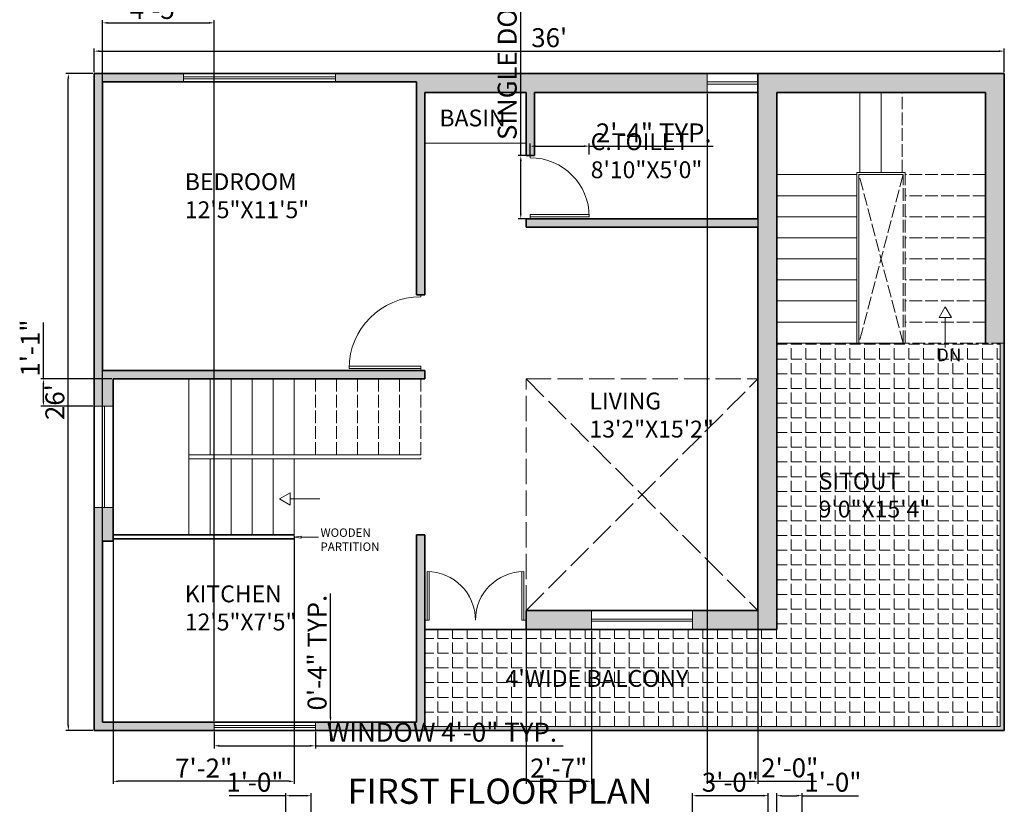
# Model space of a CAD drawing. Units: inches. Extents: x 1947 to 4744, y 610 to 1869.
# Tile 4 of 8: x 3678 to 4146, y 1074 to 1446. Entities that reach past the tile are written whole.
import ezdxf

# ---------------------------------------------------------------- set-up
doc = ezdxf.new("R2010")
doc.units = ezdxf.units.IN
doc.linetypes.add('ACAD_ISO02W100', pattern=[15, 12, -3])
for name, color, linetype, lineweight in [('A-ANNO-DIMS', 2, 'Continuous', 18), ('A-ANNO-SYMB', 2, 'Continuous', 18), ('A-ANNO-TEXT', 7, 'Continuous', 18), ('A-ANNO-TITL', 7, 'Continuous', 35), ('A-AREA-IDEN', 7, 'Continuous', 18), ('A-DOOR', 3, 'Continuous', 18), ('A-FLOR-FIXT', 9, 'Continuous', 18), ('A-FLOR-OPEN-PROJ', 8, 'ACAD_ISO02W100', 13), ('A-FLOR-STRS', 7, 'Continuous', 18), ('A-FLOR-STRS-OVHD', 7, 'ACAD_ISO02W100', 13), ('A-GLAZ', 4, 'Continuous', 18), ('A-WALL', 7, 'Continuous', 35), ('A-WALL-PRHT', 7, 'Continuous', 18)]:
    doc.layers.add(name, color=color, linetype=linetype, lineweight=lineweight)
doc.layers.add('A-FLOR-PATT', color=251, linetype='Continuous', lineweight=13, true_color=0x636466)
doc.layers.add('A-WALL-PATT', color=18, linetype='Continuous', lineweight=13, true_color=0x000000)
doc.styles.get("Standard").update_dxf_attribs({"font": 'arial.ttf'})
doc.dimstyles.new('ISO-25', dxfattribs={"dimtxt": 9, "dimasz": 2.5, "dimexe": 1.25, "dimexo": 0.625, "dimtad": 1, "dimdec": 1, "dimlunit": 3, "dimtxsty": 'Standard', "dimcen": 2.5, "dimadec": 0, "dimazin": 0, "dimtfac": 1, "dimtdec": 1, "dimtmove": 0, "dimatfit": 3, "dimfxl": 1, "dimarcsym": 0})

# ---------------------------------------------------------------- blocks, each defined once
blk = doc.blocks.new('1')
for p, q in [((4267.36, 1627.82), (4267.36, 1650.82)), ((4268.36, 1627.82), (4268.36, 1650.82)), ((4312.36, 1627.82), (4312.36, 1650.82)), ((4313.36, 1627.82), (4313.36, 1650.82)), ((4266.36, 1627.82), (4268.36, 1627.82)), ((4314.36, 1627.82), (4312.36, 1627.82))]:
    blk.add_line(p, q)
at = {"ltscale": 0.5}
for centre, start, end in [((4267.36, 1627.82), 0, 90), ((4313.36, 1627.82), 90, 180)]:
    blk.add_arc(centre, 23, start, end, dxfattribs=at)
blk = doc.blocks.new('2')
for p, q in [((4319.45, 1679.18), (4319.45, 1713.18)), ((4320.45, 1679.18), (4320.45, 1713.18)), ((4318.45, 1679.18), (4320.45, 1679.18)), ((4353.45, 1679.18), (4354.45, 1679.18))]:
    blk.add_line(p, q)
at = {"ltscale": 0.5}
blk.add_arc((4319.45, 1679.18), 34, 0, 90, dxfattribs=at)
blk = doc.blocks.new('4')
for p, q in [((3808.6, 1693.11), (3808.6, 1721.11)), ((3809.6, 1693.11), (3809.6, 1721.11)), ((3807.6, 1693.11), (3809.6, 1693.11)), ((3836.6, 1693.11), (3837.6, 1693.11))]:
    blk.add_line(p, q)
at = {"ltscale": 0.5}
blk.add_arc((3808.6, 1693.11), 28, 0, 90, dxfattribs=at)
blk = doc.blocks.new('*D7')
at = {"layer": 'A-ANNO-DIMS', "color": 0, "lineweight": -2, "transparency": 16777216}
for p, q in [((3712.91, 1420.79), (3700.04, 1420.79)), ((3701.29, 1111.29), (3701.29, 1418.29)), ((3712.91, 1108.79), (3700.04, 1108.79))]:
    blk.add_line(p, q, dxfattribs=at)
at = {"layer": 'A-ANNO-DIMS', "color": 0, "transparency": 16777216}
for points in [[(3700.88, 1418.29), (3701.71, 1418.29), (3701.29, 1420.79)], [(3700.88, 1111.29), (3701.71, 1111.29), (3701.29, 1108.79)]]:
    blk.add_solid(points, dxfattribs=at)
at = {"layer": 'Defpoints', "color": 0, "transparency": 16777216}
for p in [(3701.29, 1420.79), (3713.53, 1420.79), (3713.53, 1108.79)]:
    blk.add_point(p, dxfattribs=at)
at = {"layer": 'A-ANNO-DIMS', "color": 0, "transparency": 16777216, "insert": (3696.07, 1264.79), "char_height": 9, "attachment_point": 5, "rotation": 90}
blk.add_mtext("26'", dxfattribs=at)
blk = doc.blocks.new('*D8')
at = {"layer": 'A-ANNO-DIMS', "color": 0, "lineweight": -2, "transparency": 16777216}
for p, q in [((3713.53, 1421.41), (3713.53, 1432.67)), ((3716.03, 1431.42), (4143.03, 1431.42)), ((4145.53, 1421.41), (4145.53, 1432.67))]:
    blk.add_line(p, q, dxfattribs=at)
at = {"layer": 'A-ANNO-DIMS', "color": 0, "transparency": 16777216}
for points in [[(3716.03, 1431.83), (3716.03, 1431), (3713.53, 1431.42)], [(4143.03, 1431.83), (4143.03, 1431), (4145.53, 1431.42)]]:
    blk.add_solid(points, dxfattribs=at)
at = {"layer": 'Defpoints', "color": 0, "transparency": 16777216}
for p in [(4145.53, 1431.42), (3713.53, 1420.79), (4145.53, 1420.79)]:
    blk.add_point(p, dxfattribs=at)
at = {"layer": 'A-ANNO-DIMS', "color": 0, "transparency": 16777216, "insert": (3929.53, 1436.64), "char_height": 9, "attachment_point": 5}
blk.add_mtext("36'", dxfattribs=at)
blk = doc.blocks.new('WIN-72-4')
for p, q in [((0, 0), (0, 4)), ((72, 2.5), (0, 2.5)), ((72, 1.5), (0, 1.5)), ((72, 0), (72, 4))]:
    blk.add_line(p, q)
blk = doc.blocks.new('WIN-48-4')
for p, q in [((0, 0), (0, 4)), ((48, 2.5), (0, 2.5)), ((48, 1.5), (0, 1.5)), ((48, 0), (48, 4))]:
    blk.add_line(p, q)
blk = doc.blocks.new('WIN-48-9')
for p, q in [((0, 0), (0, 9)), ((48, 5), (0, 5)), ((48, 0), (48, 9)), ((48, 4), (0, 4))]:
    blk.add_line(p, q)
blk = doc.blocks.new('STAIR-DIRECTION')
blk.add_line((2.91, 14.18), (2.91, 0))
blk.add_lwpolyline([(2.91, 19.23), (0, 14.18), (5.83, 14.18)], close=True)
blk = doc.blocks.new('PARTITION-LEADER')
blk.add_line((3.21, 0.5), (11.48, 0.5))
blk.add_lwpolyline([(0, 0.5), (3.21, 0), (3.21, 0.99)], close=True)
blk = doc.blocks.new('*D82')
at = {"layer": 'A-ANNO-DIMS', "color": 0, "lineweight": -2, "transparency": 16777216}
for p, q in [((3916.03, 1381.79), (3916.03, 1531.18)), ((3919.91, 1381.79), (3914.78, 1381.79)), ((3916.03, 1354.29), (3916.03, 1379.29)), ((3919.91, 1351.79), (3914.78, 1351.79))]:
    blk.add_line(p, q, dxfattribs=at)
at = {"layer": 'A-ANNO-DIMS', "color": 0, "transparency": 16777216}
for points in [[(3915.61, 1379.29), (3916.45, 1379.29), (3916.03, 1381.79)], [(3915.61, 1354.29), (3916.45, 1354.29), (3916.03, 1351.79)]]:
    blk.add_solid(points, dxfattribs=at)
at = {"layer": 'Defpoints', "color": 0, "transparency": 16777216}
for p in [(3916.03, 1381.79), (3920.53, 1381.79), (3920.53, 1351.79)]:
    blk.add_point(p, dxfattribs=at)
at = {"layer": 'A-ANNO-DIMS', "color": 0, "transparency": 16777216, "insert": (3910.75, 1457.73), "char_height": 9, "attachment_point": 5, "rotation": 90}
blk.add_mtext('SINGLE DOOR 2\'-6" TYP.', dxfattribs=at)
blk = doc.blocks.new('*D83')
at = {"layer": 'A-ANNO-DIMS', "color": 0, "lineweight": -2, "transparency": 16777216}
for p, q in [((3920.53, 1382.41), (3920.53, 1387.54)), ((3923.03, 1386.29), (3946.03, 1386.29)), ((3948.53, 1382.41), (3948.53, 1387.54)), ((3948.53, 1386.29), (4007.29, 1386.29))]:
    blk.add_line(p, q, dxfattribs=at)
at = {"layer": 'A-ANNO-DIMS', "color": 0, "transparency": 16777216}
for points in [[(3923.03, 1386.71), (3923.03, 1385.87), (3920.53, 1386.29)], [(3946.03, 1386.71), (3946.03, 1385.87), (3948.53, 1386.29)]]:
    blk.add_solid(points, dxfattribs=at)
at = {"layer": 'Defpoints', "color": 0, "transparency": 16777216}
for p in [(3948.53, 1386.29), (3920.53, 1381.79), (3948.53, 1381.79)]:
    blk.add_point(p, dxfattribs=at)
at = {"layer": 'A-ANNO-DIMS', "color": 0, "transparency": 16777216, "insert": (3979.16, 1391.44), "char_height": 9, "attachment_point": 5}
blk.add_mtext('2\'-4" TYP.', dxfattribs=at)
blk = doc.blocks.new('*D90')
at = {"layer": 'A-ANNO-DIMS', "color": 0, "lineweight": -2, "transparency": 16777216}
for p, q in [((3770.53, 1108.16), (3770.53, 1100.34)), ((3818.53, 1108.16), (3818.53, 1100.34)), ((3773.03, 1101.59), (3816.03, 1101.59)), ((3818.53, 1101.59), (3936.17, 1101.59))]:
    blk.add_line(p, q, dxfattribs=at)
at = {"layer": 'A-ANNO-DIMS', "color": 0, "transparency": 16777216}
for points in [[(3773.03, 1102.01), (3773.03, 1101.17), (3770.53, 1101.59)], [(3816.03, 1102.01), (3816.03, 1101.17), (3818.53, 1101.59)]]:
    blk.add_solid(points, dxfattribs=at)
at = {"layer": 'Defpoints', "color": 0, "transparency": 16777216}
for p in [(3770.53, 1108.79), (3818.53, 1108.79), (3818.53, 1101.59)]:
    blk.add_point(p, dxfattribs=at)
at = {"layer": 'A-ANNO-DIMS', "color": 0, "transparency": 16777216, "insert": (3878.6, 1106.87), "char_height": 9, "attachment_point": 5}
blk.add_mtext('WINDOW 4\'-0" TYP.', dxfattribs=at)
blk = doc.blocks.new('*D91')
at = {"layer": 'A-ANNO-DIMS', "color": 0, "lineweight": -2, "transparency": 16777216}
for p, q in [((3825.73, 1115.29), (3825.73, 1173.9)), ((3819.16, 1112.79), (3826.98, 1112.79)), ((3825.73, 1108.79), (3825.73, 1112.79)), ((3819.16, 1108.79), (3826.98, 1108.79)), ((3825.73, 1106.29), (3825.73, 1103.79))]:
    blk.add_line(p, q, dxfattribs=at)
at = {"layer": 'A-ANNO-DIMS', "color": 0, "transparency": 16777216}
for points in [[(3825.31, 1115.29), (3826.15, 1115.29), (3825.73, 1112.79)], [(3825.31, 1106.29), (3826.15, 1106.29), (3825.73, 1108.79)]]:
    blk.add_solid(points, dxfattribs=at)
at = {"layer": 'Defpoints', "color": 0, "transparency": 16777216}
for p in [(3818.53, 1112.79), (3825.73, 1112.79), (3818.53, 1108.79)]:
    blk.add_point(p, dxfattribs=at)
at = {"layer": 'A-ANNO-DIMS', "color": 0, "transparency": 16777216, "insert": (3820.51, 1145.84), "char_height": 9, "attachment_point": 5, "rotation": 90}
blk.add_mtext('0\'-4" TYP.', dxfattribs=at)
blk = doc.blocks.new('*D108')
at = {"layer": 'A-ANNO-DIMS', "color": 0, "lineweight": -2, "transparency": 16777216}
for p, q in [((3717.53, 1113.41), (3717.53, 1446.09)), ((3720.03, 1444.84), (3768.03, 1444.84)), ((3770.53, 1113.41), (3770.53, 1446.09))]:
    blk.add_line(p, q, dxfattribs=at)
at = {"layer": 'A-ANNO-DIMS', "color": 0, "transparency": 16777216}
for points in [[(3720.03, 1445.26), (3720.03, 1444.42), (3717.53, 1444.84)], [(3768.03, 1445.26), (3768.03, 1444.42), (3770.53, 1444.84)]]:
    blk.add_solid(points, dxfattribs=at)
at = {"layer": 'Defpoints', "color": 0, "transparency": 16777216}
for p in [(3770.53, 1444.84), (3717.53, 1112.79), (3770.53, 1112.79)]:
    blk.add_point(p, dxfattribs=at)
at = {"layer": 'A-ANNO-DIMS', "color": 0, "transparency": 16777216, "insert": (3744.03, 1450.04), "char_height": 9, "attachment_point": 5}
blk.add_mtext('4\'-5"', dxfattribs=at)
blk = doc.blocks.new('*D110')
at = {"layer": 'A-ANNO-DIMS', "color": 0, "lineweight": -2, "transparency": 16777216}
for p, q in [((3997.53, 1050.49), (3997.53, 1079.17)), ((4031.03, 1077.92), (4000.03, 1077.92)), ((4033.53, 1054.49), (4033.53, 1079.17))]:
    blk.add_line(p, q, dxfattribs=at)
at = {"layer": 'A-ANNO-DIMS', "color": 0, "transparency": 16777216}
for points in [[(4000.03, 1078.33), (4000.03, 1077.5), (3997.53, 1077.92)], [(4031.03, 1078.33), (4031.03, 1077.5), (4033.53, 1077.92)]]:
    blk.add_solid(points, dxfattribs=at)
at = {"layer": 'Defpoints', "color": 0, "transparency": 16777216}
for p in [(3997.53, 1077.92), (4033.53, 1053.87), (3997.53, 1049.87)]:
    blk.add_point(p, dxfattribs=at)
at = {"layer": 'A-ANNO-DIMS', "color": 0, "transparency": 16777216, "insert": (4015.53, 1083.14), "char_height": 9, "attachment_point": 5}
blk.add_mtext('3\'-0"', dxfattribs=at)
blk = doc.blocks.new('*D113')
at = {"layer": 'A-ANNO-DIMS', "color": 0, "lineweight": -2, "transparency": 16777216}
for p, q in [((4037.53, 909.49), (4037.53, 1079.17)), ((4040.03, 1077.92), (4047.03, 1077.92)), ((4049.53, 913.49), (4049.53, 1079.17)), ((4049.53, 1077.92), (4076.36, 1077.92))]:
    blk.add_line(p, q, dxfattribs=at)
at = {"layer": 'A-ANNO-DIMS', "color": 0, "transparency": 16777216}
for points in [[(4040.03, 1078.33), (4040.03, 1077.5), (4037.53, 1077.92)], [(4047.03, 1078.33), (4047.03, 1077.5), (4049.53, 1077.92)]]:
    blk.add_solid(points, dxfattribs=at)
at = {"layer": 'Defpoints', "color": 0, "transparency": 16777216}
for p in [(4049.53, 1077.92), (4049.53, 912.87), (4037.53, 908.87)]:
    blk.add_point(p, dxfattribs=at)
at = {"layer": 'A-ANNO-DIMS', "color": 0, "transparency": 16777216, "insert": (4064.19, 1083.14), "char_height": 9, "attachment_point": 5}
blk.add_mtext('1\'-0"', dxfattribs=at)
blk = doc.blocks.new('*D114')
at = {"layer": 'A-ANNO-DIMS', "color": 0, "lineweight": -2, "transparency": 16777216}
for p, q in [((3804.53, 1077.92), (3777.7, 1077.92)), ((3804.53, 790.49), (3804.53, 1079.17)), ((3814.03, 1077.92), (3807.03, 1077.92)), ((3816.53, 790.49), (3816.53, 1079.17))]:
    blk.add_line(p, q, dxfattribs=at)
at = {"layer": 'A-ANNO-DIMS', "color": 0, "transparency": 16777216}
for points in [[(3807.03, 1078.33), (3807.03, 1077.5), (3804.53, 1077.92)], [(3814.03, 1078.33), (3814.03, 1077.5), (3816.53, 1077.92)]]:
    blk.add_solid(points, dxfattribs=at)
at = {"layer": 'Defpoints', "color": 0, "transparency": 16777216}
for p in [(3804.53, 1077.92), (3804.53, 789.87), (3816.53, 789.87)]:
    blk.add_point(p, dxfattribs=at)
at = {"layer": 'A-ANNO-DIMS', "color": 0, "transparency": 16777216, "insert": (3789.87, 1083.14), "char_height": 9, "attachment_point": 5}
blk.add_mtext('1\'-0"', dxfattribs=at)
blk = doc.blocks.new('*D115')
at = {"layer": 'A-ANNO-DIMS', "color": 0, "lineweight": -2, "transparency": 16777216}
for p, q in [((3722.53, 1201.16), (3722.53, 1083.49)), ((3808.53, 1201.16), (3808.53, 1083.49)), ((3806.03, 1084.74), (3725.03, 1084.74))]:
    blk.add_line(p, q, dxfattribs=at)
at = {"layer": 'A-ANNO-DIMS', "color": 0, "transparency": 16777216}
for points in [[(3725.03, 1085.16), (3725.03, 1084.32), (3722.53, 1084.74)], [(3806.03, 1085.16), (3806.03, 1084.32), (3808.53, 1084.74)]]:
    blk.add_solid(points, dxfattribs=at)
at = {"layer": 'Defpoints', "color": 0, "transparency": 16777216}
for p in [(3722.53, 1201.79), (3808.53, 1201.79), (3722.53, 1084.74)]:
    blk.add_point(p, dxfattribs=at)
at = {"layer": 'A-ANNO-DIMS', "color": 0, "transparency": 16777216, "insert": (3765.53, 1089.88), "char_height": 9, "attachment_point": 5}
blk.add_mtext('7\'-2"', dxfattribs=at)
blk = doc.blocks.new('*D116')
at = {"layer": 'A-ANNO-DIMS', "color": 0, "lineweight": -2, "transparency": 16777216}
for p, q in [((3689.48, 1275.79), (3689.48, 1302.62)), ((3721.91, 1275.79), (3688.23, 1275.79)), ((3689.48, 1265.29), (3689.48, 1273.29)), ((3712.91, 1262.79), (3688.23, 1262.79))]:
    blk.add_line(p, q, dxfattribs=at)
at = {"layer": 'A-ANNO-DIMS', "color": 0, "transparency": 16777216}
for points in [[(3689.06, 1273.29), (3689.9, 1273.29), (3689.48, 1275.79)], [(3689.06, 1265.29), (3689.9, 1265.29), (3689.48, 1262.79)]]:
    blk.add_solid(points, dxfattribs=at)
at = {"layer": 'Defpoints', "color": 0, "transparency": 16777216}
for p in [(3689.48, 1275.79), (3722.53, 1275.79), (3713.53, 1262.79)]:
    blk.add_point(p, dxfattribs=at)
at = {"layer": 'A-ANNO-DIMS', "color": 0, "transparency": 16777216, "insert": (3684.34, 1290.45), "char_height": 9, "attachment_point": 5, "rotation": 90}
blk.add_mtext('1\'-1"', dxfattribs=at)
blk = doc.blocks.new('*D119')
at = {"layer": 'A-ANNO-DIMS', "color": 0, "lineweight": -2, "transparency": 16777216}
for p, q in [((4004.53, 1411.16), (4004.53, 1083.49)), ((4028.53, 1411.16), (4028.53, 1083.49)), ((4007.03, 1084.74), (4026.03, 1084.74)), ((4028.53, 1084.74), (4056.36, 1084.74))]:
    blk.add_line(p, q, dxfattribs=at)
at = {"layer": 'A-ANNO-DIMS', "color": 0, "transparency": 16777216}
for points in [[(4007.03, 1085.16), (4007.03, 1084.32), (4004.53, 1084.74)], [(4026.03, 1085.16), (4026.03, 1084.32), (4028.53, 1084.74)]]:
    blk.add_solid(points, dxfattribs=at)
at = {"layer": 'Defpoints', "color": 0, "transparency": 16777216}
for p in [(4004.53, 1411.79), (4028.53, 1411.79), (4028.53, 1084.74)]:
    blk.add_point(p, dxfattribs=at)
at = {"layer": 'A-ANNO-DIMS', "color": 0, "transparency": 16777216, "insert": (4043.69, 1089.96), "char_height": 9, "attachment_point": 5}
blk.add_mtext('2\'-0"', dxfattribs=at)
blk = doc.blocks.new('*D120')
at = {"layer": 'A-ANNO-DIMS', "color": 0, "lineweight": -2, "transparency": 16777216}
for p, q in [((3918.53, 1156.16), (3918.53, 1083.49)), ((3949.53, 1156.16), (3949.53, 1083.49)), ((3921.03, 1084.74), (3947.03, 1084.74))]:
    blk.add_line(p, q, dxfattribs=at)
at = {"layer": 'A-ANNO-DIMS', "color": 0, "transparency": 16777216}
for points in [[(3921.03, 1085.16), (3921.03, 1084.32), (3918.53, 1084.74)], [(3947.03, 1085.16), (3947.03, 1084.32), (3949.53, 1084.74)]]:
    blk.add_solid(points, dxfattribs=at)
at = {"layer": 'Defpoints', "color": 0, "transparency": 16777216}
for p in [(3918.53, 1156.79), (3949.53, 1156.79), (3949.53, 1084.74)]:
    blk.add_point(p, dxfattribs=at)
at = {"layer": 'A-ANNO-DIMS', "color": 0, "transparency": 16777216, "insert": (3934.03, 1089.88), "char_height": 9, "attachment_point": 5}
blk.add_mtext('2\'-7"', dxfattribs=at)

msp = doc.modelspace()

# ---------------------------------------------------------------- hatches: boundary and pattern name
at = {"layer": 'A-FLOR-PATT'}
h = msp.add_hatch(dxfattribs=at)
h.set_pattern_fill('ANGLE', color=256)
h.set_pattern_definition([(0, (0, 0), (0, 6.985), [5.08, -1.905]), (90, (0, 0), (-6.985, 4e-16), [5.08, -1.905])])
h.paths.add_polyline_path([(4037.53, 1156.79), (3870.53, 1156.79), (3870.53, 1110.79), (4143.53, 1110.79), (4143.53, 1292.79), (4097.53, 1292.79), (4037.53, 1292.79)])
h.paths.add_polyline_path([(4111.9, 1280.8), (4127.69, 1280.8), (4127.69, 1293.61), (4111.9, 1293.61)], flags=9)
h.paths.add_polyline_path([(3906.66, 1125.02), (4009.57, 1125.02), (4009.57, 1142.1), (3906.66, 1142.1)], flags=24)
h.paths.add_polyline_path([(4054.68, 1205.44), (4110.92, 1205.44), (4110.92, 1235.86), (4054.68, 1235.86)], flags=24)
at = {"layer": 'A-WALL-PATT'}
h = msp.add_hatch(color=256, dxfattribs=at)
h.dxf.hatch_style = 1
h.paths.add_polyline_path([(3870.53, 1279.79), (3717.53, 1279.79), (3717.53, 1416.79), (3756.03, 1416.79), (3756.03, 1420.79), (3713.53, 1420.79), (3713.53, 1262.79), (3722.53, 1262.79), (3722.53, 1275.79), (3870.53, 1275.79)])
h.paths.add_polyline_path([(3722.53, 1214.79), (3713.53, 1214.79), (3713.53, 1108.79), (3770.53, 1108.79), (3770.53, 1112.79), (3717.53, 1112.79), (3717.53, 1198.79), (3722.53, 1198.79)])
h.paths.add_polyline_path([(3870.53, 1201.79), (3866.53, 1201.79), (3866.53, 1112.79), (3818.53, 1112.79), (3818.53, 1108.79), (3870.53, 1108.79)])
h.paths.add_polyline_path([(3949.53, 1165.79), (3918.53, 1165.79), (3918.53, 1156.79), (3949.53, 1156.79)])
h.paths.add_polyline_path([(4037.53, 1411.79), (4136.53, 1411.79), (4136.53, 1292.79), (4145.53, 1292.79), (4145.53, 1420.79), (4028.53, 1420.79), (4028.53, 1351.79), (3918.53, 1351.79), (3918.53, 1347.79), (4028.53, 1347.79), (4028.53, 1165.79), (3997.53, 1165.79), (3997.53, 1156.79), (4037.53, 1156.79)])
h.paths.add_polyline_path([(4004.53, 1420.79), (3828.03, 1420.79), (3828.03, 1416.79), (3866.53, 1416.79), (3866.53, 1315.79), (3870.53, 1315.79), (3870.53, 1411.79), (3918.53, 1411.79), (3918.53, 1381.79), (3922.53, 1381.79), (3922.53, 1411.79), (4004.53, 1411.79)])
h.paths.add_polyline_path([(4145.53, 1292.79), (4143.53, 1292.79), (4143.53, 1110.79), (4145.53, 1110.79)])
h.paths.add_polyline_path([(4143.53, 1110.79), (3870.53, 1110.79), (3870.53, 1108.79), (4143.53, 1108.79)])
h.paths.add_polyline_path([(4145.53, 1110.79), (4143.53, 1110.79), (4143.53, 1108.79), (4145.53, 1108.79)])

# ---------------------------------------------------------------- linework, layer by layer
at = {"layer": 'A-FLOR-FIXT'}
msp.add_line((3918.53, 1387.79), (3870.53, 1387.79), dxfattribs=at)
at = {"layer": 'A-FLOR-OPEN-PROJ'}
for p, q in [((3918.53, 1275.79), (4028.53, 1165.79)), ((3918.53, 1165.79), (4028.53, 1275.79))]:
    msp.add_line(p, q, dxfattribs=at)
msp.add_lwpolyline([(4028.53, 1165.79), (3918.53, 1165.79), (3918.53, 1275.79), (4028.53, 1275.79)], close=True, dxfattribs=at)
at = {"layer": 'A-FLOR-STRS'}
for p, q in [((4077.03, 1373.79), (4077.03, 1411.79)), ((4087.03, 1373.79), (4087.03, 1411.79)), ((4075.53, 1372.79), (4037.53, 1372.79)), ((4098.53, 1373.79), (4075.53, 1373.79)), ((4075.53, 1292.79), (4075.53, 1373.79)), ((4097.53, 1372.79), (4076.53, 1372.79)), ((4076.53, 1292.79), (4076.53, 1372.79)), ((4075.53, 1362.79), (4037.53, 1362.79)), ((4075.53, 1352.79), (4037.53, 1352.79)), ((4075.53, 1342.79), (4037.53, 1342.79)), ((4075.53, 1332.79), (4037.53, 1332.79)), ((4075.53, 1322.79), (4037.53, 1322.79)), ((4075.53, 1312.79), (4037.53, 1312.79)), ((4075.53, 1302.79), (4037.53, 1302.79)), ((4097.53, 1292.79), (4037.53, 1292.79)), ((3758.53, 1275.79), (3758.53, 1201.79)), ((3768.53, 1275.79), (3768.53, 1239.79)), ((3778.53, 1275.79), (3778.53, 1239.79)), ((3788.53, 1275.79), (3788.53, 1239.79)), ((3798.53, 1275.79), (3798.53, 1239.79)), ((3808.53, 1275.79), (3808.53, 1239.79)), ((3868.53, 1239.79), (3758.53, 1239.79)), ((3758.53, 1237.79), (3868.53, 1237.79)), ((3768.53, 1237.79), (3768.53, 1201.79)), ((3778.53, 1237.79), (3778.53, 1201.79)), ((3788.53, 1237.79), (3788.53, 1201.79)), ((3798.53, 1237.79), (3798.53, 1201.79)), ((3808.53, 1237.79), (3808.53, 1199.79))]:
    msp.add_line(p, q, dxfattribs=at)
at = {"layer": 'A-FLOR-STRS-OVHD', "ltscale": 0.5}
for p, q in [((4097.03, 1373.79), (4097.03, 1411.79)), ((4097.53, 1372.79), (4076.53, 1292.79)), ((4097.53, 1292.79), (4076.53, 1372.79)), ((4097.53, 1292.79), (4097.53, 1372.79)), ((4098.53, 1292.79), (4098.53, 1373.79)), ((4136.53, 1372.79), (4098.53, 1372.79)), ((4136.53, 1362.79), (4098.53, 1362.79)), ((4136.53, 1352.79), (4098.53, 1352.79)), ((4136.53, 1342.79), (4098.53, 1342.79)), ((4136.53, 1332.79), (4098.53, 1332.79)), ((4136.53, 1322.79), (4098.53, 1322.79)), ((4136.53, 1312.79), (4098.53, 1312.79)), ((4136.53, 1302.79), (4098.53, 1302.79)), ((4145.53, 1292.79), (4097.53, 1292.79)), ((3818.53, 1275.79), (3818.53, 1239.79)), ((3828.53, 1275.79), (3828.53, 1239.79)), ((3838.53, 1275.79), (3838.53, 1239.79)), ((3848.53, 1275.79), (3848.53, 1239.79)), ((3858.53, 1275.79), (3858.53, 1239.79)), ((3868.53, 1275.79), (3868.53, 1237.79))]:
    msp.add_line(p, q, dxfattribs=at)
at = {"layer": 'A-GLAZ'}
for p, q in [((4004.53, 1411.79), (4004.53, 1420.79)), ((4028.53, 1416.79), (4004.53, 1416.79)), ((4028.53, 1415.79), (4004.53, 1415.79))]:
    msp.add_line(p, q, dxfattribs=at)
at = {"layer": 'A-WALL'}
for p, q in [((4145.53, 1420.79), (3713.53, 1420.79)), ((3713.53, 1420.79), (3713.53, 1108.79)), ((4028.53, 1351.79), (4028.53, 1420.79)), ((4145.53, 1108.79), (4145.53, 1420.79)), ((3866.53, 1416.79), (3717.53, 1416.79)), ((3717.53, 1416.79), (3717.53, 1279.79)), ((3866.53, 1416.79), (3866.53, 1315.79)), ((3918.53, 1411.79), (3870.53, 1411.79)), ((3870.53, 1411.79), (3870.53, 1315.79)), ((3918.53, 1381.79), (3918.53, 1411.79)), ((4028.53, 1411.79), (3922.53, 1411.79)), ((3922.53, 1381.79), (3922.53, 1411.79)), ((4136.53, 1411.79), (4037.53, 1411.79)), ((4037.53, 1156.79), (4037.53, 1411.79)), ((4136.53, 1292.79), (4136.53, 1411.79)), ((3922.53, 1381.79), (3918.53, 1381.79)), ((4028.53, 1351.79), (3918.53, 1351.79)), ((3918.53, 1347.79), (3918.53, 1351.79)), ((3918.53, 1347.79), (4028.53, 1347.79)), ((4028.53, 1165.79), (4028.53, 1347.79)), ((3870.53, 1315.79), (3866.53, 1315.79)), ((3870.53, 1279.79), (3717.53, 1279.79)), ((3870.53, 1279.79), (3870.53, 1275.79)), ((3870.53, 1275.79), (3722.53, 1275.79)), ((3722.53, 1275.79), (3722.53, 1198.79)), ((3722.53, 1201.79), (3808.53, 1201.79)), ((3866.53, 1201.79), (3866.53, 1112.79)), ((3866.53, 1201.79), (3870.53, 1201.79)), ((3870.53, 1201.79), (3870.53, 1108.79)), ((3717.53, 1198.79), (3717.53, 1112.79)), ((3717.53, 1198.79), (3722.53, 1198.79)), ((3722.53, 1199.79), (3808.53, 1199.79)), ((3918.53, 1165.79), (3918.53, 1156.79)), ((3918.53, 1165.79), (4028.53, 1165.79)), ((3870.53, 1156.79), (4037.53, 1156.79)), ((3717.53, 1112.79), (3866.53, 1112.79)), ((3713.53, 1108.79), (4145.53, 1108.79))]:
    msp.add_line(p, q, dxfattribs=at)
at = {"layer": 'A-WALL-PRHT'}
for p, q in [((4143.53, 1110.79), (4143.53, 1292.79)), ((3870.53, 1110.79), (4143.53, 1110.79))]:
    msp.add_line(p, q, dxfattribs=at)

# ---------------------------------------------------------------- block references
at = {"layer": 'A-ANNO-SYMB'}
msp.add_blockref('STAIR-DIRECTION', (4114.62, 1290.71), dxfattribs=at)
at = {"layer": 'A-ANNO-SYMB', "rotation": 90.00000000000095}
msp.add_blockref('STAIR-DIRECTION', (3820.7, 1215.88), dxfattribs=at)
at = {"layer": 'A-ANNO-TEXT'}
msp.add_blockref('PARTITION-LEADER', (3808.53, 1200.17), dxfattribs=at)
at = {"layer": 'A-DOOR', "xscale": -1, "rotation": 270}
msp.add_blockref('4', (2227.42, -2455.81), dxfattribs=at)
at = {"layer": 'A-DOOR', "rotation": 90.00000000000003}
msp.add_blockref('2', (5547.71, -3038.66), dxfattribs=at)
at = {"layer": 'A-DOOR'}
msp.add_blockref('1', (-395.83, -466.53), dxfattribs=at)
at = {"layer": 'A-GLAZ'}
for name, p in [('WIN-72-4', (3756.03, 1416.79)), ('WIN-48-9', (3949.53, 1156.79)), ('WIN-48-4', (3770.53, 1108.79))]:
    msp.add_blockref(name, p, dxfattribs=at)
at = {"layer": 'A-GLAZ', "rotation": 270.0000000000002}
msp.add_blockref('WIN-48-9', (3713.53, 1262.79), dxfattribs=at)

# ---------------------------------------------------------------- texts
at = {"layer": 'A-ANNO-TEXT', "attachment_point": 1}
for s, insert, char_height in [('{\\fTimes New Roman|b0|i0|c0|p18;BASIN}', (3877.42, 1403.67), 8), ('{\\fTimes New Roman|b0|i0|c0|p18;DN}', (4113.55, 1290.21), 6), ('{\\fTimes New Roman|b0|i0|c0|p18;WOODEN\\PPARTITION}', (3820.99, 1204.8), 4)]:
    msp.add_mtext_dynamic_manual_height_columns(s, width=158.3328, gutter_width=12.5, heights=[0], dxfattribs=dict(at, insert=insert, char_height=char_height))
at = {"layer": 'A-ANNO-TITL', "insert": (3833.83, 1086.05), "char_height": 12, "attachment_point": 1}
msp.add_mtext_dynamic_manual_height_columns('{\\fTimes New Roman|b0|i0|c0|p18;FIRST FLOOR PLAN}', width=253.4596, gutter_width=12.5, heights=[0], dxfattribs=at)
at = {"layer": 'A-AREA-IDEN', "char_height": 8, "attachment_point": 1}
for s, width, heights, insert in [('{\\fTimes New Roman|b0|i0|c0|p18;C.TOILET\\P8\'10"X5\'0"}', 64.3566, [21.47], (3949.23, 1392.43)), ('{\\fTimes New Roman|b0|i0|c0|p18;BEDROOM\\P12\'5"X11\'5"}', 64.3566, [0], (3756.58, 1373.44)), ('{\\fTimes New Roman|b0|i0|c0|p18;LIVING\\P13\'2"X15\'2"}', 64.3566, [21.47], (3948.63, 1269.3)), ('{\\fTimes New Roman|b0|i0|c0|p18;SITOUT\\P9\'0"X15\'4"}', 64.3566, [0], (4057.42, 1231.33)), ('{\\fTimes New Roman|b0|i0|c0|p18;KITCHEN\\P12\'5"X7\'5"}', 64.3566, [0], (3756.58, 1177.74)), ("{\\fTimes New Roman|b0|i0|c0|p18;4'WIDE BALCONY}", 158.3328, [0], (3908.84, 1137.58))]:
    msp.add_mtext_dynamic_manual_height_columns(s, width=width, gutter_width=12.5, heights=heights, dxfattribs=dict(at, insert=insert))

# ---------------------------------------------------------------- dimensions: what is measured, and where the dimension line sits
at = {"layer": 'A-ANNO-DIMS'}
for base, p1, p2, text, picture, middle in [((3916.03, 1381.79), (3920.53, 1351.79), (3920.53, 1381.79), 'SINGLE DOOR <> TYP.', '*D82', (3910.75, 1457.73)), ((3825.73, 1112.79), (3818.53, 1108.79), (3818.53, 1112.79), '<> TYP.', '*D91', (3820.51, 1145.84))]:
    dim = msp.add_linear_dim(base=base, p1=p1, p2=p2, angle=90, text=text, dimstyle='ISO-25', override={"dimdec": 1, "dimlfac": 1, "dimrnd": 0, "dimzin": 1, "dimdsep": 46, "dimlunit": 4, "dimfrac": 2}, dxfattribs=at)
    dim.commit()
    dim.dimension.update_dxf_attribs({"geometry": picture, "text_midpoint": middle})
for base, p1, p2, override, picture, middle in [((3770.53, 1444.84), (3717.53, 1112.79), (3770.53, 1112.79), {"dimdec": 1, "dimlfac": 1, "dimrnd": 0, "dimzin": 1, "dimdsep": 46, "dimlunit": 4, "dimfrac": 2}, '*D108', (3744.03, 1450.04)), ((4145.53, 1431.42), (3713.53, 1420.79), (4145.53, 1420.79), {"dimclrd": 0, "dimclre": 0, "dimclrt": 0}, '*D8', (3929.53, 1436.64)), ((4028.53, 1084.74), (4004.53, 1411.79), (4028.53, 1411.79), {"dimdec": 1, "dimlfac": 1, "dimrnd": 0, "dimzin": 1, "dimdsep": 46, "dimlunit": 4, "dimfrac": 2}, '*D119', (4043.69, 1089.96)), ((3722.53, 1084.74), (3808.53, 1201.79), (3722.53, 1201.79), {"dimdec": 1, "dimlfac": 1, "dimrnd": 0, "dimzin": 1, "dimdsep": 46, "dimlunit": 4, "dimfrac": 2}, '*D115', (3765.53, 1089.88)), ((3949.53, 1084.74), (3918.53, 1156.79), (3949.53, 1156.79), {"dimdec": 1, "dimlfac": 1, "dimrnd": 0, "dimzin": 1, "dimdsep": 46, "dimlunit": 4, "dimfrac": 2}, '*D120', (3934.03, 1089.88)), ((3804.53, 1077.92), (3816.53, 789.87), (3804.53, 789.87), {"dimdec": 1, "dimlfac": 1, "dimrnd": 0, "dimzin": 1, "dimdsep": 46, "dimlunit": 4, "dimfrac": 2}, '*D114', (3789.87, 1083.14)), ((3997.53, 1077.92), (4033.53, 1053.87), (3997.53, 1049.87), {"dimdec": 1, "dimlfac": 1, "dimrnd": 0, "dimzin": 1, "dimdsep": 46, "dimlunit": 4, "dimfrac": 2}, '*D110', (4015.53, 1083.14)), ((4049.53, 1077.92), (4037.53, 908.87), (4049.53, 912.87), {"dimdec": 1, "dimlfac": 1, "dimrnd": 0, "dimzin": 1, "dimdsep": 46, "dimlunit": 4, "dimfrac": 2}, '*D113', (4064.19, 1083.14))]:
    dim = msp.add_linear_dim(base=base, p1=p1, p2=p2, dimstyle='ISO-25', override=override, dxfattribs=at)
    dim.commit()
    dim.dimension.update_dxf_attribs({"geometry": picture, "text_midpoint": middle})
for base, p1, p2, override, picture, middle in [((3701.29, 1420.79), (3713.53, 1108.79), (3713.53, 1420.79), {"dimclrd": 0, "dimclre": 0, "dimclrt": 0}, '*D7', (3696.07, 1264.79)), ((3689.48, 1275.79), (3713.53, 1262.79), (3722.53, 1275.79), {"dimdec": 1, "dimlfac": 1, "dimrnd": 0, "dimzin": 1, "dimdsep": 46, "dimlunit": 4, "dimfrac": 2}, '*D116', (3684.34, 1290.45))]:
    dim = msp.add_linear_dim(base=base, p1=p1, p2=p2, angle=90, dimstyle='ISO-25', override=override, dxfattribs=at)
    dim.commit()
    dim.dimension.update_dxf_attribs({"geometry": picture, "text_midpoint": middle})
for base, p1, p2, text, picture, middle in [((3948.53, 1386.29), (3920.53, 1381.79), (3948.53, 1381.79), '<> TYP.', '*D83', (3979.16, 1391.44)), ((3818.53, 1101.59), (3770.53, 1108.79), (3818.53, 1108.79), 'WINDOW <> TYP.', '*D90', (3878.6, 1106.87))]:
    dim = msp.add_linear_dim(base=base, p1=p1, p2=p2, text=text, dimstyle='ISO-25', override={"dimdec": 1, "dimlfac": 1, "dimrnd": 0, "dimzin": 1, "dimdsep": 46, "dimlunit": 4, "dimfrac": 2}, dxfattribs=at)
    dim.commit()
    dim.dimension.update_dxf_attribs({"geometry": picture, "text_midpoint": middle})

doc.saveas('drawing.dxf')
